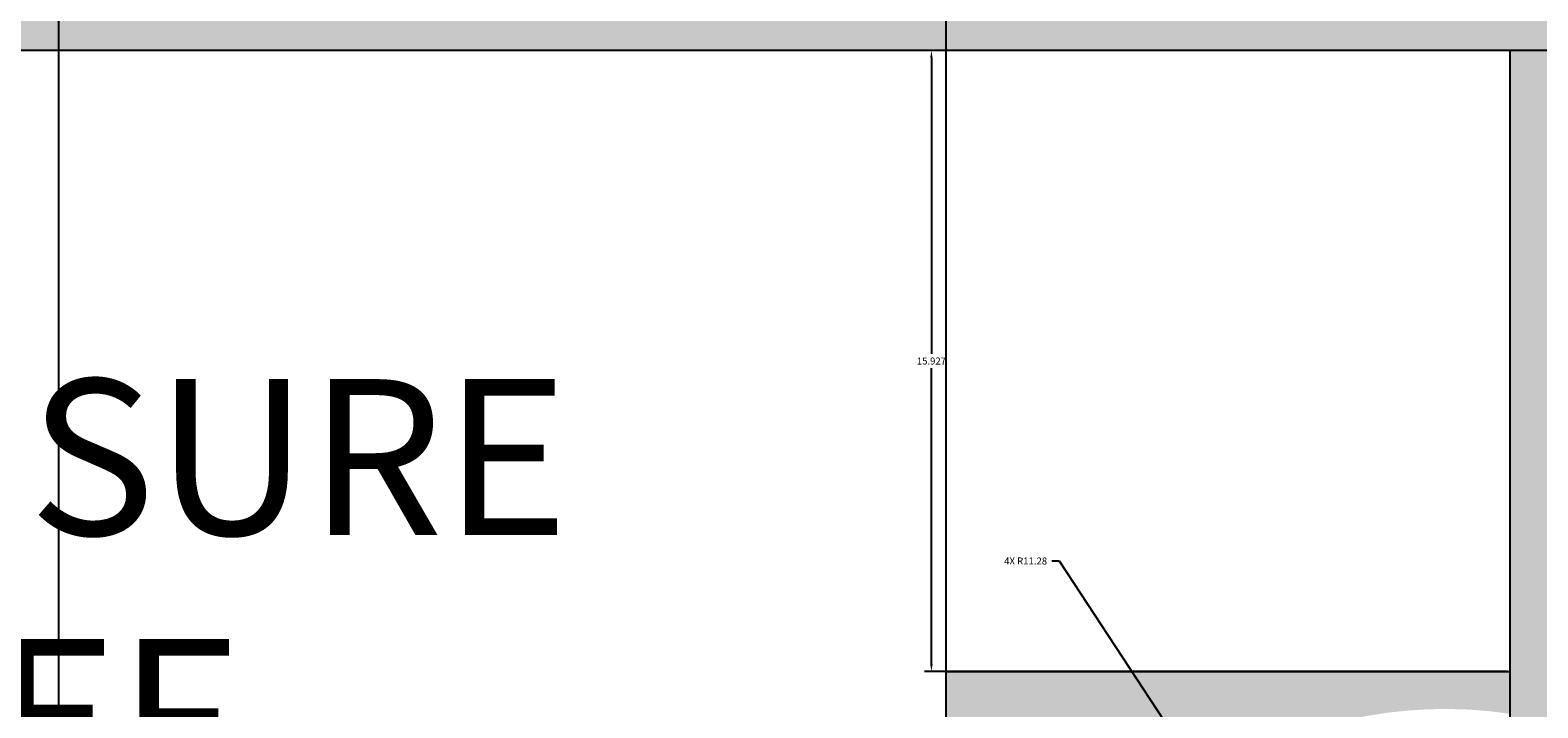
# Model space of a CAD drawing. Units: millimetres. Extents: x -11 to 280, y -4 to 208.
# Tile 31 of 55: x 150 to 189, y 88 to 106. Entities that reach past the tile are written whole.
import ezdxf

# ---------------------------------------------------------------- set-up
doc = ezdxf.new("R2010")
doc.units = ezdxf.units.MM
for name, color, linetype, lineweight in [('M-ANNO-TEXT', 7, 'Continuous', 18), ('M-DIMS', 2, 'Continuous', 18), ('M-HYDR-PRES', 7, 'Continuous', 25), ('M-HYDR-VALV', 7, 'Continuous', 25), ('M-HYDR-VALV-PATT', 252, 'Continuous', 13)]:
    doc.layers.add(name, color=color, linetype=linetype, lineweight=lineweight)
doc.layers.add('M-HYDR-PRES-PATT', color=240, linetype='Continuous', lineweight=13, true_color=0xed1f24)
doc.styles.get("Standard").update_dxf_attribs({"font": 'arial.ttf'})
doc.dimstyles.get("Standard").update_dxf_attribs({"dimtxt": 0.18, "dimasz": 0.18, "dimexe": 0.18, "dimexo": 0.0625, "dimgap": 0.09, "dimtad": 0, "dimtih": 1, "dimtoh": 1, "dimdec": 4, "dimzin": 0, "dimdsep": 46, "dimtxsty": 'Standard', "dimcen": 0.09, "dimadec": 0, "dimazin": 0, "dimtfac": 1, "dimtdec": 4, "dimtofl": 0, "dimtmove": 0, "dimatfit": 3, "dimfxl": 1, "dimtolj": 1, "dimtzin": 0, "dimarcsym": 0})

# ---------------------------------------------------------------- blocks, each defined once
blk = doc.blocks.new('*D5')
at = {"layer": 'Defpoints', "color": 0, "transparency": 16777216}
for p in [(24.759, 192.645), (-10.087, 11.435), (261.686, 11.435)]:
    blk.add_point(p, dxfattribs=at)
at = {"layer": 'M-DIMS', "color": 0, "lineweight": -2, "transparency": 16777216}
for p, q in [((24.696, 192.645), (-10.267, 192.645)), ((-10.087, 192.465), (-10.087, 102.222)), ((-10.087, 11.615), (-10.087, 101.858)), ((261.624, 11.435), (-10.267, 11.435))]:
    blk.add_line(p, q, dxfattribs=at)
at = {"layer": 'M-DIMS', "color": 0, "transparency": 16777216}
for points in [[(-10.117, 192.465), (-10.057, 192.465), (-10.087, 192.645)], [(-10.117, 11.615), (-10.057, 11.615), (-10.087, 11.435)]]:
    blk.add_solid(points, dxfattribs=at)
at = {"layer": 'M-DIMS', "color": 0, "transparency": 16777216, "insert": (-10.087, 102.04), "char_height": 0.18, "attachment_point": 5}
blk.add_mtext('\\A1;181.2', dxfattribs=at)
blk = doc.blocks.new('*D12')
at = {"layer": 'Defpoints', "color": 0, "transparency": 16777216}
for p in [(173.804, 207.495), (118.514, 96.485), (173.804, 89.387)]:
    blk.add_point(p, dxfattribs=at)
at = {"layer": 'M-DIMS', "color": 0, "lineweight": -2, "transparency": 16777216}
for p, q in [((118.514, 96.547), (118.514, 207.675)), ((118.694, 207.495), (145.765, 207.495)), ((173.624, 207.495), (146.553, 207.495)), ((173.804, 89.45), (173.804, 207.675))]:
    blk.add_line(p, q, dxfattribs=at)
at = {"layer": 'M-DIMS', "color": 0, "transparency": 16777216}
for points in [[(118.694, 207.525), (118.694, 207.465), (118.514, 207.495)], [(173.624, 207.525), (173.624, 207.465), (173.804, 207.495)]]:
    blk.add_solid(points, dxfattribs=at)
at = {"layer": 'M-DIMS', "color": 0, "transparency": 16777216, "insert": (146.159, 207.495), "char_height": 0.18, "attachment_point": 5}
blk.add_mtext('\\A1;55.29', dxfattribs=at)
blk = doc.blocks.new('*D17')
at = {"layer": 'Defpoints', "color": 0, "transparency": 16777216}
for p in [(173.424, 105.314), (188.274, 105.314), (188.274, 89.387)]:
    blk.add_point(p, dxfattribs=at)
at = {"layer": 'M-DIMS', "color": 0, "lineweight": -2, "transparency": 16777216}
for p, q in [((188.212, 105.314), (173.244, 105.314)), ((173.424, 105.134), (173.424, 97.533)), ((173.424, 89.567), (173.424, 97.169)), ((188.212, 89.387), (173.244, 89.387))]:
    blk.add_line(p, q, dxfattribs=at)
at = {"layer": 'M-DIMS', "color": 0, "transparency": 16777216}
for points in [[(173.394, 105.134), (173.454, 105.134), (173.424, 105.314)], [(173.394, 89.567), (173.454, 89.567), (173.424, 89.387)]]:
    blk.add_solid(points, dxfattribs=at)
at = {"layer": 'M-DIMS', "color": 0, "transparency": 16777216, "insert": (173.424, 97.351), "char_height": 0.18, "attachment_point": 5}
blk.add_mtext('\\A1;15.927', dxfattribs=at)
blk = doc.blocks.new('*D18')
at = {"layer": 'Defpoints', "color": 0, "transparency": 16777216}
for p in [(173.804, 207.495), (173.804, 65.064), (151.022, 43.599)]:
    blk.add_point(p, dxfattribs=at)
at = {"layer": 'M-DIMS', "color": 0, "lineweight": -2, "transparency": 16777216}
for p, q in [((151.022, 43.662), (151.022, 207.675)), ((151.202, 207.495), (162.017, 207.495)), ((173.624, 207.495), (162.808, 207.495)), ((173.804, 65.126), (173.804, 207.675))]:
    blk.add_line(p, q, dxfattribs=at)
at = {"layer": 'M-DIMS', "color": 0, "transparency": 16777216}
for points in [[(151.202, 207.525), (151.202, 207.465), (151.022, 207.495)], [(173.624, 207.525), (173.624, 207.465), (173.804, 207.495)]]:
    blk.add_solid(points, dxfattribs=at)
at = {"layer": 'M-DIMS', "color": 0, "transparency": 16777216, "insert": (162.413, 207.495), "char_height": 0.18, "attachment_point": 5}
blk.add_mtext('\\A1;22.78', dxfattribs=at)
blk = doc.blocks.new('*D20')
at = {"layer": 'Defpoints', "color": 0, "transparency": 16777216}
for p in [(231.68, 207.495), (151.022, 43.599), (231.68, 43.599)]:
    blk.add_point(p, dxfattribs=at)
at = {"layer": 'M-DIMS', "color": 0, "lineweight": -2, "transparency": 16777216}
for p, q in [((151.022, 43.662), (151.022, 207.675)), ((151.202, 207.495), (190.957, 207.495)), ((231.5, 207.495), (191.745, 207.495)), ((231.68, 43.662), (231.68, 207.675))]:
    blk.add_line(p, q, dxfattribs=at)
at = {"layer": 'M-DIMS', "color": 0, "transparency": 16777216}
for points in [[(151.202, 207.525), (151.202, 207.465), (151.022, 207.495)], [(231.5, 207.525), (231.5, 207.465), (231.68, 207.495)]]:
    blk.add_solid(points, dxfattribs=at)
at = {"layer": 'M-DIMS', "color": 0, "transparency": 16777216, "insert": (191.351, 207.495), "char_height": 0.18, "attachment_point": 5}
blk.add_mtext('\\A1;80.66', dxfattribs=at)
blk = doc.blocks.new('*D29')
at = {"layer": 'Defpoints', "color": 0, "transparency": 16777216}
for p in [(180.42, 86.567), (186.62, 77.144)]:
    blk.add_point(p, dxfattribs=at)
at = {"layer": 'M-DIMS', "color": 0, "lineweight": -2, "transparency": 16777216}
for p, q in [((176.52, 92.221), (176.7, 92.221)), ((176.7, 92.221), (180.321, 86.718)), ((186.53, 77.144), (186.71, 77.144)), ((186.62, 77.054), (186.62, 77.234))]:
    blk.add_line(p, q, dxfattribs=at)
at = {"layer": 'M-DIMS', "color": 0, "transparency": 16777216}
blk.add_solid([(180.346, 86.734), (180.296, 86.701), (180.42, 86.567)], dxfattribs=at)
at = {"layer": 'M-DIMS', "color": 0, "transparency": 16777216, "insert": (175.843, 92.221), "char_height": 0.18, "attachment_point": 5}
blk.add_mtext('\\A1;4X R11.28', dxfattribs=at)

msp = doc.modelspace()

# ---------------------------------------------------------------- hatches: boundary and pattern name
at = {"layer": 'M-HYDR-PRES-PATT'}
h = msp.add_hatch(color=256, dxfattribs=at)
h.set_gradient(color1=(237, 31, 36), color2=(237, 31, 36), tint=1)
h.paths.add_polyline_path([(232.2, 133.1228), (228.7, 133.1228), (228.7, 108.8141), (102.7646, 108.8141), (102.7646, 105.3141), (232.2, 105.3141)])
h.paths.add_polyline_path([(128.8433, 105.3141), (125.3433, 105.3141), (125.3433, 91.7099, 1), (128.8433, 91.7099)])
h.paths.add_polyline_path([(229.1617, 78.7098), (196.7745, 78.7098, -0.4142136), (191.7745, 83.7098), (191.7745, 105.3141), (188.2745, 105.3141), (188.2745, 80.2098, 0.4142136), (193.2745, 75.2098), (225.6617, 75.2098), (225.6617, 43.5991), (229.1617, 43.5991)])
h.paths.add_polyline_path([(102.7646, 110.3704), (95.5776, 110.3704), (95.5776, 103.9022), (102.7646, 103.9022)])
h.paths.add_polyline_path([(100.7059, 107.2502), (99.1711, 106.3641), (99.1711, 106.8641), (97.1711, 106.8641), (97.1711, 107.6363), (99.1711, 107.6363), (99.1711, 108.1363)], flags=16)
h.paths.add_polyline_path([(234.6119, 138.4081), (226.5106, 138.4081), (226.5106, 133.1228), (234.6119, 133.1228)])
h.paths.add_polyline_path([(231.1963, 135.7055), (230.2965, 134.1786), (229.4241, 135.7213), (229.9241, 135.7168), (229.9418, 137.7167), (230.7141, 137.7099), (230.6963, 135.71)], flags=16)
at = {"layer": 'M-HYDR-VALV-PATT'}
h = msp.add_hatch(color=256, dxfattribs=at)
h.set_gradient(color1=(153, 27, 30), color2=(153, 27, 30), tint=1)
h.paths.add_polyline_path([(131.8437, 88.2421, -0.3394543), (132.5849, 89.208), (121.2548, 86.1721, -0.4931454), (122.5137, 85.2062, -0.3394543), (121.7725, 84.2403), (133.1025, 87.2762, -0.4931454)])
h.paths.add_polyline_path([(133.1025, 83.1351, -0.4931454), (131.8437, 84.101, -0.3394543), (132.5849, 85.0669), (121.2548, 82.031, -0.4931454), (122.5137, 81.0651, -0.3394543), (121.7725, 80.0992)])
h.paths.add_polyline_path([(133.1025, 78.994, -0.4931454), (131.8437, 79.9599, -0.3394543), (132.5849, 80.9258), (121.2548, 77.8899, -0.4931454), (122.5137, 76.924, -0.3394543), (121.7725, 75.9581)])
h.paths.add_polyline_path([(197.7905, 78.7098), (200.0003, 78.7098), (200.0003, 89.3873), (191.7745, 89.3873), (191.7745, 87.1776, -0.2439164)])
h.paths.add_polyline_path([(200.0003, 65.0638), (200.0003, 75.2098), (197.7325, 75.2098, -0.4135811), (184.7092, 66.0277), (184.7092, 65.0638)])
h.paths.add_polyline_path([(181.2092, 65.0638), (181.2092, 67.2471, -0.2598454), (175.3563, 76.54), (173.8038, 76.54), (173.8038, 65.0638)])
h.paths.add_polyline_path([(188.2745, 88.3022), (188.2745, 89.3873), (173.8038, 89.3873), (173.8038, 80.04), (175.7181, 80.04, -0.3816661)])

# ---------------------------------------------------------------- linework, layer by layer
at = {"layer": 'M-HYDR-PRES'}
msp.add_lwpolyline([(232.2, 133.1228), (232.2, 105.3141), (102.7646, 105.3141)], dxfattribs=at)
msp.add_lwpolyline([(188.2745, 105.3141), (188.2745, 80.2098, 0.4142136), (193.2745, 75.2098), (225.6617, 75.2098), (225.6617, 43.5991)], format="xyb", dxfattribs=at)
at = {"layer": 'M-HYDR-VALV'}
msp.add_lwpolyline([(173.8038, 80.04), (173.8038, 89.3873), (188.2745, 89.3873)], dxfattribs=at)

# ---------------------------------------------------------------- texts
at = {"layer": 'M-ANNO-TEXT', "insert": (136.8574, 96.8862), "char_height": 4, "attachment_point": 1}
msp.add_mtext_dynamic_manual_height_columns('PRESSURE\\P RELIEF\\PVALVE', width=63.617875, gutter_width=12.5, heights=[0], dxfattribs=at)

# ---------------------------------------------------------------- dimensions: what is measured, and where the dimension line sits
at = {"layer": 'M-DIMS'}
for base, p1, p2, picture, middle in [((173.8038, 207.495), (118.5137, 96.4849), (173.8038, 89.3873), '*D12', (146.1587, 207.495)), ((173.8038, 207.495), (151.0217, 43.5991), (173.8038, 65.0638), '*D18', (162.4127, 207.495)), ((231.6803, 207.495), (151.0217, 43.5991), (231.6803, 43.5991), '*D20', (191.351, 207.495))]:
    dim = msp.add_linear_dim(base=base, p1=p1, p2=p2, dimstyle='Standard', override={"dimdec": 2, "dimlfac": 1, "dimrnd": 0, "dimzin": 0, "dimdsep": 46, "dimlunit": 2}, dxfattribs=at)
    dim.commit()
    dim.dimension.update_dxf_attribs({"geometry": picture, "text_midpoint": middle})
for base, p1, p2, override, picture, middle in [((-10.0865, 11.4346), (24.7588, 192.645), (261.6863, 11.4346), {"dimdec": 1, "dimlfac": 1, "dimrnd": 0, "dimzin": 0, "dimdsep": 46, "dimlunit": 2}, '*D5', (-10.0865, 102.0398)), ((173.4245, 105.3141), (188.2745, 89.3873), (188.2745, 105.3141), {"dimdec": 3, "dimlfac": 1, "dimrnd": 0, "dimzin": 0, "dimdsep": 46, "dimlunit": 2}, '*D17', (173.4245, 97.3507))]:
    dim = msp.add_linear_dim(base=base, p1=p1, p2=p2, angle=90, dimstyle='Standard', override=override, dxfattribs=at)
    dim.commit()
    dim.dimension.update_dxf_attribs({"geometry": picture, "text_midpoint": middle})
dim = msp.add_radius_dim(center=(186.6199, 77.1445), mpoint=(180.4197, 86.5674), text='4X <>', dimstyle='Standard', override={"dimdec": 2, "dimlfac": 1, "dimrnd": 0, "dimzin": 0, "dimdsep": 46, "dimlunit": 2}, dxfattribs=at)
dim.commit()
dim.dimension.update_dxf_attribs({"geometry": '*D29', "text_midpoint": (175.8426, 92.2211), "dimtype": 164})

doc.saveas('drawing.dxf')
